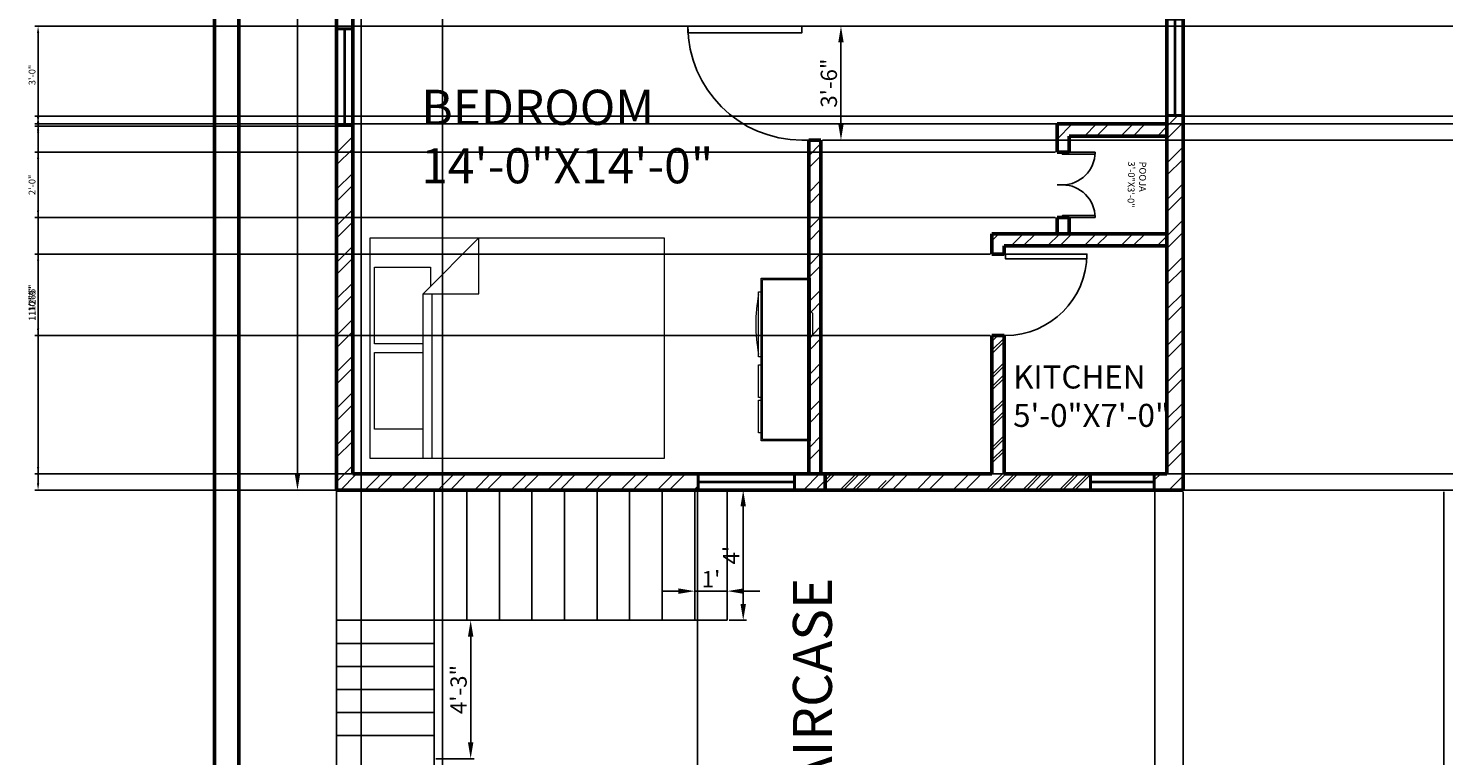
# Model space of a CAD drawing. Units: inches. Extents: x -12550 to 6516, y 1273 to 18700.
# Tile 4 of 19: x 1904 to 2426, y 1958 to 2226. Entities that reach past the tile are written whole.
import ezdxf

# ---------------------------------------------------------------- set-up
doc = ezdxf.new("R2010")
doc.units = ezdxf.units.IN
for name, color, linetype, lineweight in [('A-ANNO-DIMS', 2, 'Continuous', 18), ('A-AREA-IDEN', 1, 'Continuous', 18), ('A-DOOR', 5, 'Continuous', 25), ('A-FLOR-STRS', 6, 'Continuous', 25), ('A-FURN', 8, 'Continuous', 18), ('A-GLAZ', 3, 'Continuous', 25), ('A-WALL', 7, 'Continuous', 50), ('A-WALL-PATT', 8, 'Continuous', 13)]:
    doc.layers.add(name, color=color, linetype=linetype, lineweight=lineweight)
doc.styles.get("Standard").update_dxf_attribs({"font": 'arial.ttf'})
doc.dimstyles.new('ISO-25', dxfattribs={"dimtxt": 2.5, "dimasz": 2.5, "dimexe": 1.25, "dimexo": 0.625, "dimtad": 1, "dimlunit": 4, "dimtxsty": 'Standard', "dimcen": 2.5, "dimadec": 0, "dimazin": 0, "dimtfac": 1, "dimtmove": 0, "dimatfit": 3, "dimfxl": 1, "dimarcsym": 0})
pattern_1 = [(45, (-2e-13, 567), (-6.735192, 6.735192), []), (45, (4.49, 567), (-6.735192, 6.735192), [])]

# ---------------------------------------------------------------- blocks, each defined once
blk = doc.blocks.new('*U2')
for p, q in [((0, 0), (0, -5)), ((30, 0), (30, -5))]:
    blk.add_line(p, q)
blk.add_lwpolyline([(0, 0), (0, 30), (1.75, 30), (1.75, 0)], close=True)
blk.add_arc((0, 0), 30, 0, 90)
blk = doc.blocks.new('Bed - Queen')
for p, q in [((0, -80.00003), (0, 0)), ((0, 0), (59.99999, 0)), ((59.99999, 0), (59.99999, -80.00003)), ((7.99999, -1.2), (28.79998, -1.2)), ((7.99999, -14.4), (7.99999, -1.2)), ((28.79998, -1.2), (28.79998, -14.4)), ((31.19999, -1.2), (51.99999, -1.2)), ((31.19999, -14.4), (31.19999, -1.2)), ((51.99999, -1.2), (51.99999, -16.4)), ((0, -14.4), (44.8, -14.4)), ((59.99999, -29.6), (44.8, -14.4)), ((44.8, -14.4), (44.8, -29.6)), ((44.8, -16.8), (0, -16.8)), ((51.99999, -16.4), (46.79936, -16.4)), ((44.8, -29.6), (59.99999, -29.6)), ((59.99999, -80.00003), (0, -80.00003))]:
    blk.add_line(p, q)
blk = doc.blocks.new('Entertainment Center')
for p, q in [((-4, 0), (-5, -1)), ((4, 0), (-4, 0)), ((5, -1), (4, 0)), ((-17, -19), (-17, -1)), ((-17, -1), (43, -1)), ((-16.5, -18.5), (-16.5, -1.5)), ((-16.5, -1.5), (42.5, -1.5)), ((42.5, -1.5), (42.5, -18.5)), ((43, -1), (43, -19)), ((43, -19), (-17, -19)), ((42.5, -18.5), (-16.5, -18.5)), ((-12, -20), (-12, -19)), ((12, -20), (-12, -20)), ((12, -19), (12, -20)), ((15, -20), (15, -19)), ((27, -20), (15, -20)), ((27, -19), (27, -20)), ((28, -20), (28, -19)), ((40, -20), (28, -20)), ((40, -19), (40, -20))]:
    blk.add_line(p, q)
blk.add_arc((0, 40), 61, 259.6111, 280.3889)
blk = doc.blocks.new('*D10')
at = {"layer": 'A-ANNO-DIMS', "color": 0, "lineweight": -2, "transparency": 16777216}
for p, q in [((2196.81, 2227.25), (2204.82, 2227.25)), ((2203.57, 2221.25), (2203.57, 2191.25)), ((2196.81, 2185.25), (2204.82, 2185.25))]:
    blk.add_line(p, q, dxfattribs=at)
at = {"layer": 'A-ANNO-DIMS', "color": 0, "transparency": 16777216}
for points in [[(2202.57, 2221.25), (2204.57, 2221.25), (2203.57, 2227.25)], [(2202.57, 2191.25), (2204.57, 2191.25), (2203.57, 2185.25)]]:
    blk.add_solid(points, dxfattribs=at)
at = {"layer": 'Defpoints', "color": 0, "transparency": 16777216}
for p in [(2196.19, 2227.25), (2196.19, 2185.25), (2203.57, 2185.25)]:
    blk.add_point(p, dxfattribs=at)
at = {"layer": 'A-ANNO-DIMS', "color": 0, "transparency": 16777216, "insert": (2199.88, 2206.25), "char_height": 6, "attachment_point": 5, "rotation": 90}
blk.add_mtext('3\'-6"', dxfattribs=at)
blk = doc.blocks.new('*D11')
at = {"layer": 'A-ANNO-DIMS', "color": 0, "lineweight": -2, "transparency": 16777216}
for p, q in [((2162.31, 2056.25), (2168.79, 2056.25)), ((2167.54, 2014.25), (2167.54, 2050.25)), ((2162.31, 2008.25), (2168.79, 2008.25))]:
    blk.add_line(p, q, dxfattribs=at)
at = {"layer": 'A-ANNO-DIMS', "color": 0, "transparency": 16777216}
for points in [[(2166.54, 2050.25), (2168.54, 2050.25), (2167.54, 2056.25)], [(2166.54, 2014.25), (2168.54, 2014.25), (2167.54, 2008.25)]]:
    blk.add_solid(points, dxfattribs=at)
at = {"layer": 'Defpoints', "color": 0, "transparency": 16777216}
for p in [(2161.69, 2056.25), (2167.54, 2056.25), (2161.69, 2008.25)]:
    blk.add_point(p, dxfattribs=at)
at = {"layer": 'A-ANNO-DIMS', "color": 0, "transparency": 16777216, "insert": (2163.92, 2032.25), "char_height": 6, "attachment_point": 5, "rotation": 90}
blk.add_mtext("4'", dxfattribs=at)
blk = doc.blocks.new('*D12')
at = {"layer": 'A-ANNO-DIMS', "color": 0, "lineweight": -2, "transparency": 16777216}
for p, q in [((2143.69, 2019.01), (2137.69, 2019.01)), ((2149.69, 2008.87), (2149.69, 2020.26)), ((2161.69, 2019.01), (2149.69, 2019.01)), ((2161.69, 2008.87), (2161.69, 2020.26)), ((2167.69, 2019.01), (2173.69, 2019.01))]:
    blk.add_line(p, q, dxfattribs=at)
at = {"layer": 'A-ANNO-DIMS', "color": 0, "transparency": 16777216}
for points in [[(2143.69, 2020.01), (2143.69, 2018.01), (2149.69, 2019.01)], [(2167.69, 2020.01), (2167.69, 2018.01), (2161.69, 2019.01)]]:
    blk.add_solid(points, dxfattribs=at)
at = {"layer": 'Defpoints', "color": 0, "transparency": 16777216}
for p in [(2149.69, 2019.01), (2149.69, 2008.25), (2161.69, 2008.25)]:
    blk.add_point(p, dxfattribs=at)
at = {"layer": 'A-ANNO-DIMS', "color": 0, "transparency": 16777216, "insert": (2155.69, 2022.65), "char_height": 6, "attachment_point": 5}
blk.add_mtext("1'", dxfattribs=at)
blk = doc.blocks.new('*D13')
at = {"layer": 'A-ANNO-DIMS', "color": 0, "lineweight": -2, "transparency": 16777216}
for p, q in [((2054.31, 2008.25), (2068.36, 2008.25)), ((2067.11, 2002.25), (2067.11, 1963.25)), ((2054.31, 1957.25), (2068.36, 1957.25))]:
    blk.add_line(p, q, dxfattribs=at)
at = {"layer": 'A-ANNO-DIMS', "color": 0, "transparency": 16777216}
for points in [[(2066.11, 2002.25), (2068.11, 2002.25), (2067.11, 2008.25)], [(2066.11, 1963.25), (2068.11, 1963.25), (2067.11, 1957.25)]]:
    blk.add_solid(points, dxfattribs=at)
at = {"layer": 'Defpoints', "color": 0, "transparency": 16777216}
for p in [(2053.69, 2008.25), (2053.69, 1957.25), (2067.11, 1957.25)]:
    blk.add_point(p, dxfattribs=at)
at = {"layer": 'A-ANNO-DIMS', "color": 0, "transparency": 16777216, "insert": (2063.42, 1982.75), "char_height": 6, "attachment_point": 5, "rotation": 90}
blk.add_mtext('4\'-3"', dxfattribs=at)
blk = doc.blocks.new('*D15')
at = {"layer": 'A-ANNO-DIMS', "color": 0, "lineweight": -2, "transparency": 16777216}
for p, q in [((2017.06, 2473.25), (2002.03, 2473.25)), ((2003.28, 2467.25), (2003.28, 2062.25)), ((2017.06, 2056.25), (2002.03, 2056.25))]:
    blk.add_line(p, q, dxfattribs=at)
at = {"layer": 'A-ANNO-DIMS', "color": 0, "transparency": 16777216}
for points in [[(2002.28, 2467.25), (2004.28, 2467.25), (2003.28, 2473.25)], [(2002.28, 2062.25), (2004.28, 2062.25), (2003.28, 2056.25)]]:
    blk.add_solid(points, dxfattribs=at)
at = {"layer": 'Defpoints', "color": 0, "transparency": 16777216}
for p in [(2017.69, 2473.25), (2003.28, 2056.25), (2017.69, 2056.25)]:
    blk.add_point(p, dxfattribs=at)
at = {"layer": 'A-ANNO-DIMS', "color": 0, "transparency": 16777216, "insert": (1999.59, 2264.75), "char_height": 6, "attachment_point": 5, "rotation": 90}
blk.add_mtext('34\'-9"', dxfattribs=at)
blk = doc.blocks.new('WIN-3FT')
for p, q in [((0, 0), (0, 6)), ((0, 6), (36.02, 6)), ((0.5, 0), (0.5, 6)), ((35.52, 6), (35.52, 0)), ((36.02, 6), (36.02, 0)), ((36.02, 0), (0, 0)), ((35.52, 3.2), (0.5, 3.2)), ((35.52, 2.8), (0.5, 2.8))]:
    blk.add_line(p, q)
blk = doc.blocks.new('WIN-2FT')
for p, q in [((0, 0), (0, 24.02)), ((0, 24.02), (6, 24.02)), ((0, 23.52), (6, 23.52)), ((2.8, 0.5), (2.8, 23.52)), ((3.2, 0.5), (3.2, 23.52)), ((6, 24.02), (6, 0)), ((6, 0.5), (0, 0.5)), ((6, 0), (0, 0))]:
    blk.add_line(p, q)
blk = doc.blocks.new('*D133')
at = {"layer": 'A-ANNO-DIMS', "color": 0, "lineweight": -2, "transparency": 16777216}
for p, q in [((2017.06, 2190.44), (1906.44, 2190.44)), ((1907.69, 2058.75), (1907.69, 2187.94)), ((2017.06, 2056.25), (1906.44, 2056.25))]:
    blk.add_line(p, q, dxfattribs=at)
at = {"layer": 'A-ANNO-DIMS', "color": 0, "transparency": 16777216}
for points in [[(1907.27, 2187.94), (1908.11, 2187.94), (1907.69, 2190.44)], [(1907.27, 2058.75), (1908.11, 2058.75), (1907.69, 2056.25)]]:
    blk.add_solid(points, dxfattribs=at)
at = {"layer": 'Defpoints', "color": 0, "transparency": 16777216}
for p in [(1907.69, 2190.44), (2017.69, 2190.44), (2017.69, 2056.25)]:
    blk.add_point(p, dxfattribs=at)
at = {"layer": 'A-ANNO-DIMS', "color": 0, "transparency": 16777216, "insert": (1905.81, 2123.34), "char_height": 2.5, "attachment_point": 5, "rotation": 90}
blk.add_mtext('11\'-2"', dxfattribs=at)
blk = doc.blocks.new('*D136')
at = {"layer": 'A-ANNO-DIMS', "color": 0, "lineweight": -2, "transparency": 16777216}
for p, q in [((2017.69, 2055.62), (2017.69, 1378)), ((2150.64, 2055.62), (2150.64, 1378)), ((2020.19, 1379.25), (2148.14, 1379.25))]:
    blk.add_line(p, q, dxfattribs=at)
at = {"layer": 'A-ANNO-DIMS', "color": 0, "transparency": 16777216}
for points in [[(2020.19, 1379.66), (2020.19, 1378.83), (2017.69, 1379.25)], [(2148.14, 1379.66), (2148.14, 1378.83), (2150.64, 1379.25)]]:
    blk.add_solid(points, dxfattribs=at)
at = {"layer": 'Defpoints', "color": 0, "transparency": 16777216}
for p in [(2017.69, 2056.25), (2150.64, 2056.25), (2150.64, 1379.25)]:
    blk.add_point(p, dxfattribs=at)
at = {"layer": 'A-ANNO-DIMS', "color": 0, "transparency": 16777216, "insert": (2084.16, 1381.13), "char_height": 2.5, "attachment_point": 5}
blk.add_mtext('11\'-1"', dxfattribs=at)
blk = doc.blocks.new('*D137')
at = {"layer": 'A-ANNO-DIMS', "color": 0, "lineweight": -2, "transparency": 16777216}
for p, q in [((2319.29, 2055.62), (2319.29, 1378)), ((2329.69, 2055.62), (2329.69, 1378)), ((2321.79, 1379.25), (2327.19, 1379.25)), ((2329.69, 1379.25), (2347.85, 1379.25))]:
    blk.add_line(p, q, dxfattribs=at)
at = {"layer": 'A-ANNO-DIMS', "color": 0, "transparency": 16777216}
for points in [[(2321.79, 1379.66), (2321.79, 1378.83), (2319.29, 1379.25)], [(2327.19, 1379.66), (2327.19, 1378.83), (2329.69, 1379.25)]]:
    blk.add_solid(points, dxfattribs=at)
at = {"layer": 'Defpoints', "color": 0, "transparency": 16777216}
for p in [(2319.29, 2056.25), (2329.69, 2056.25), (2329.69, 1379.25)]:
    blk.add_point(p, dxfattribs=at)
at = {"layer": 'A-ANNO-DIMS', "color": 0, "transparency": 16777216, "insert": (2340.02, 1381.16), "char_height": 2.5, "attachment_point": 5}
blk.add_mtext('0\'-10 1/2"', dxfattribs=at)
blk = doc.blocks.new('*D138')
at = {"layer": 'A-ANNO-DIMS', "color": 0, "lineweight": -2, "transparency": 16777216}
for p, q in [((2196.81, 2185.25), (2848.94, 2185.25)), ((2847.69, 2064.75), (2847.69, 2182.75)), ((2196.81, 2062.25), (2848.94, 2062.25))]:
    blk.add_line(p, q, dxfattribs=at)
at = {"layer": 'A-ANNO-DIMS', "color": 0, "transparency": 16777216}
for points in [[(2847.27, 2182.75), (2848.11, 2182.75), (2847.69, 2185.25)], [(2847.27, 2064.75), (2848.11, 2064.75), (2847.69, 2062.25)]]:
    blk.add_solid(points, dxfattribs=at)
at = {"layer": 'Defpoints', "color": 0, "transparency": 16777216}
for p in [(2196.19, 2185.25), (2847.69, 2185.25), (2196.19, 2062.25)]:
    blk.add_point(p, dxfattribs=at)
at = {"layer": 'A-ANNO-DIMS', "color": 0, "transparency": 16777216, "insert": (2845.79, 2123.75), "char_height": 2.5, "attachment_point": 5, "rotation": 90}
blk.add_mtext('10\'-3"', dxfattribs=at)
blk = doc.blocks.new('*D142')
at = {"layer": 'A-ANNO-DIMS', "color": 0, "lineweight": -2, "transparency": 16777216}
for p, q in [((2026.69, 2234.12), (2026.69, 1378)), ((2056.69, 2234.12), (2056.69, 1378)), ((2029.19, 1379.25), (2054.19, 1379.25))]:
    blk.add_line(p, q, dxfattribs=at)
at = {"layer": 'A-ANNO-DIMS', "color": 0, "transparency": 16777216}
for points in [[(2029.19, 1379.66), (2029.19, 1378.83), (2026.69, 1379.25)], [(2054.19, 1379.66), (2054.19, 1378.83), (2056.69, 1379.25)]]:
    blk.add_solid(points, dxfattribs=at)
at = {"layer": 'Defpoints', "color": 0, "transparency": 16777216}
for p in [(2026.69, 2234.75), (2056.69, 2234.75), (2056.69, 1379.25)]:
    blk.add_point(p, dxfattribs=at)
at = {"layer": 'A-ANNO-DIMS', "color": 0, "transparency": 16777216, "insert": (2041.69, 1381.15), "char_height": 2.5, "attachment_point": 5}
blk.add_mtext('2\'-6"', dxfattribs=at)
blk = doc.blocks.new('*D145')
at = {"layer": 'A-ANNO-DIMS', "color": 0, "lineweight": -2, "transparency": 16777216}
for p, q in [((2330.31, 2194.03), (2848.94, 2194.03)), ((2847.69, 2058.75), (2847.69, 2191.53)), ((2330.31, 2056.25), (2848.94, 2056.25))]:
    blk.add_line(p, q, dxfattribs=at)
at = {"layer": 'A-ANNO-DIMS', "color": 0, "transparency": 16777216}
for points in [[(2847.27, 2191.53), (2848.11, 2191.53), (2847.69, 2194.03)], [(2847.27, 2058.75), (2848.11, 2058.75), (2847.69, 2056.25)]]:
    blk.add_solid(points, dxfattribs=at)
at = {"layer": 'Defpoints', "color": 0, "transparency": 16777216}
for p in [(2329.69, 2194.03), (2847.69, 2194.03), (2329.69, 2056.25)]:
    blk.add_point(p, dxfattribs=at)
at = {"layer": 'A-ANNO-DIMS', "color": 0, "transparency": 16777216, "insert": (2845.79, 2125.14), "char_height": 2.5, "attachment_point": 5, "rotation": 90}
blk.add_mtext('11\'-6"', dxfattribs=at)
blk = doc.blocks.new('*D147')
at = {"layer": 'A-ANNO-DIMS', "color": 0, "lineweight": -2, "transparency": 16777216}
for p, q in [((2258.56, 2143.25), (1906.44, 2143.25)), ((1907.69, 2115.75), (1907.69, 2140.75)), ((2258.56, 2113.25), (1906.44, 2113.25))]:
    blk.add_line(p, q, dxfattribs=at)
at = {"layer": 'A-ANNO-DIMS', "color": 0, "transparency": 16777216}
for points in [[(1907.27, 2140.75), (1908.11, 2140.75), (1907.69, 2143.25)], [(1907.27, 2115.75), (1908.11, 2115.75), (1907.69, 2113.25)]]:
    blk.add_solid(points, dxfattribs=at)
at = {"layer": 'Defpoints', "color": 0, "transparency": 16777216}
for p in [(1907.69, 2143.25), (2259.19, 2143.25), (2259.19, 2113.25)]:
    blk.add_point(p, dxfattribs=at)
at = {"layer": 'A-ANNO-DIMS', "color": 0, "transparency": 16777216, "insert": (1905.79, 2128.25), "char_height": 2.5, "attachment_point": 5, "rotation": 90}
blk.add_mtext('2\'-6"', dxfattribs=at)
blk = doc.blocks.new('*D148')
at = {"layer": 'A-ANNO-DIMS', "color": 0, "lineweight": -2, "transparency": 16777216}
for p, q in [((2282.56, 2180.75), (1906.44, 2180.75)), ((1907.69, 2159.25), (1907.69, 2178.25)), ((2282.56, 2156.75), (1906.44, 2156.75))]:
    blk.add_line(p, q, dxfattribs=at)
at = {"layer": 'A-ANNO-DIMS', "color": 0, "transparency": 16777216}
for points in [[(1907.27, 2178.25), (1908.11, 2178.25), (1907.69, 2180.75)], [(1907.27, 2159.25), (1908.11, 2159.25), (1907.69, 2156.75)]]:
    blk.add_solid(points, dxfattribs=at)
at = {"layer": 'Defpoints', "color": 0, "transparency": 16777216}
for p in [(1907.69, 2180.75), (2283.19, 2180.75), (2283.19, 2156.75)]:
    blk.add_point(p, dxfattribs=at)
at = {"layer": 'A-ANNO-DIMS', "color": 0, "transparency": 16777216, "insert": (1905.79, 2168.75), "char_height": 2.5, "attachment_point": 5, "rotation": 90}
blk.add_mtext('2\'-0"', dxfattribs=at)
blk = doc.blocks.new('*D152')
at = {"layer": 'A-ANNO-DIMS', "color": 0, "lineweight": -2, "transparency": 16777216}
for p, q in [((2425.69, 2055.62), (2425.69, 1378)), ((2500.53, 2055.62), (2500.53, 1378)), ((2428.19, 1379.25), (2498.03, 1379.25))]:
    blk.add_line(p, q, dxfattribs=at)
at = {"layer": 'A-ANNO-DIMS', "color": 0, "transparency": 16777216}
for points in [[(2428.19, 1379.66), (2428.19, 1378.83), (2425.69, 1379.25)], [(2498.03, 1379.66), (2498.03, 1378.83), (2500.53, 1379.25)]]:
    blk.add_solid(points, dxfattribs=at)
at = {"layer": 'Defpoints', "color": 0, "transparency": 16777216}
for p in [(2425.69, 2056.25), (2500.53, 2056.25), (2500.53, 1379.25)]:
    blk.add_point(p, dxfattribs=at)
at = {"layer": 'A-ANNO-DIMS', "color": 0, "transparency": 16777216, "insert": (2463.11, 1381.15), "char_height": 2.5, "attachment_point": 5}
blk.add_mtext('6\'-3"', dxfattribs=at)
blk = doc.blocks.new('*D157')
at = {"layer": 'A-ANNO-DIMS', "color": 0, "lineweight": -2, "transparency": 16777216}
for p, q in [((2558.56, 2191.25), (1906.44, 2191.25)), ((1907.69, 2064.75), (1907.69, 2188.75)), ((2558.56, 2062.25), (1906.44, 2062.25))]:
    blk.add_line(p, q, dxfattribs=at)
at = {"layer": 'A-ANNO-DIMS', "color": 0, "transparency": 16777216}
for points in [[(1907.27, 2188.75), (1908.11, 2188.75), (1907.69, 2191.25)], [(1907.27, 2064.75), (1908.11, 2064.75), (1907.69, 2062.25)]]:
    blk.add_solid(points, dxfattribs=at)
at = {"layer": 'Defpoints', "color": 0, "transparency": 16777216}
for p in [(1907.69, 2191.25), (2559.19, 2191.25), (2559.19, 2062.25)]:
    blk.add_point(p, dxfattribs=at)
at = {"layer": 'A-ANNO-DIMS', "color": 0, "transparency": 16777216, "insert": (1905.79, 2126.75), "char_height": 2.5, "attachment_point": 5, "rotation": 90}
blk.add_mtext('10\'-9"', dxfattribs=at)
blk = doc.blocks.new('*D158')
at = {"layer": 'A-ANNO-DIMS', "color": 0, "lineweight": -2, "transparency": 16777216}
for p, q in [((2558.56, 2227.25), (1906.44, 2227.25)), ((1907.69, 2193.75), (1907.69, 2224.75)), ((2558.56, 2191.25), (1906.44, 2191.25))]:
    blk.add_line(p, q, dxfattribs=at)
at = {"layer": 'A-ANNO-DIMS', "color": 0, "transparency": 16777216}
for points in [[(1907.27, 2224.75), (1908.11, 2224.75), (1907.69, 2227.25)], [(1907.27, 2193.75), (1908.11, 2193.75), (1907.69, 2191.25)]]:
    blk.add_solid(points, dxfattribs=at)
at = {"layer": 'Defpoints', "color": 0, "transparency": 16777216}
for p in [(1907.69, 2227.25), (2559.19, 2227.25), (2559.19, 2191.25)]:
    blk.add_point(p, dxfattribs=at)
at = {"layer": 'A-ANNO-DIMS', "color": 0, "transparency": 16777216, "insert": (1905.79, 2209.25), "char_height": 2.5, "attachment_point": 5, "rotation": 90}
blk.add_mtext('3\'-0"', dxfattribs=at)
blk = doc.blocks.new('*D165')
at = {"layer": 'A-ANNO-DIMS', "color": 0, "lineweight": -2, "transparency": 16777216}
for p, q in [((2425.06, 2194.03), (1906.44, 2194.03)), ((1907.69, 2058.75), (1907.69, 2191.53)), ((2425.06, 2056.25), (1906.44, 2056.25))]:
    blk.add_line(p, q, dxfattribs=at)
at = {"layer": 'A-ANNO-DIMS', "color": 0, "transparency": 16777216}
for points in [[(1907.27, 2191.53), (1908.11, 2191.53), (1907.69, 2194.03)], [(1907.27, 2058.75), (1908.11, 2058.75), (1907.69, 2056.25)]]:
    blk.add_solid(points, dxfattribs=at)
at = {"layer": 'Defpoints', "color": 0, "transparency": 16777216}
for p in [(1907.69, 2194.03), (2425.69, 2194.03), (2425.69, 2056.25)]:
    blk.add_point(p, dxfattribs=at)
at = {"layer": 'A-ANNO-DIMS', "color": 0, "transparency": 16777216, "insert": (1905.79, 2125.14), "char_height": 2.5, "attachment_point": 5, "rotation": 90}
blk.add_mtext('11\'-6"', dxfattribs=at)

msp = doc.modelspace()

# ---------------------------------------------------------------- hatches: boundary and pattern name
at = {"layer": 'A-WALL-PATT'}
h = msp.add_hatch(dxfattribs=at)
h.set_pattern_fill('ANSI32', color=256)
h.set_pattern_definition(pattern_1)
h.paths.add_polyline_path([(2023.689, 2255.449), (2017.689, 2255.449), (2017.689, 2226.453), (2023.689, 2226.453), (2023.689, 2230.247), (2026.689, 2230.247), (2026.689, 2234.747), (2023.689, 2234.747)])
h = msp.add_hatch(dxfattribs=at)
h.set_pattern_fill('ANSI32', color=256)
h.set_pattern_definition(pattern_1)
h.paths.add_polyline_path([(2323.689, 2191.247), (2283.189, 2191.247), (2283.189, 2180.747), (2285.189, 2180.747), (2287.689, 2180.747), (2287.689, 2186.747), (2323.689, 2186.747)])
h = msp.add_hatch(dxfattribs=at)
h.set_pattern_fill('ANSI32', color=256)
h.set_pattern_definition(pattern_1)
h.paths.add_polyline_path([(2329.689, 2194.032), (2323.689, 2194.032), (2323.689, 2062.247), (2319.294, 2062.247), (2319.294, 2056.247), (2329.689, 2056.247)])
h = msp.add_hatch(dxfattribs=at)
h.set_pattern_fill('ANSI32', color=256)
h.set_pattern_definition(pattern_1)
h.paths.add_polyline_path([(2023.689, 2190.435), (2017.689, 2190.435), (2017.689, 2056.247), (2150.64, 2056.247), (2150.64, 2062.247), (2023.689, 2062.247)])
h = msp.add_hatch(dxfattribs=at)
h.set_pattern_fill('ANSI32', color=256)
h.set_pattern_definition(pattern_1)
h.paths.add_polyline_path([(2196.189, 2185.247), (2191.689, 2185.247), (2191.689, 2134.365), (2192.189, 2134.365), (2192.189, 2122.365), (2193.189, 2121.365), (2193.189, 2113.365), (2192.189, 2112.365), (2192.189, 2074.365), (2191.689, 2062.247), (2196.189, 2062.247)])
h = msp.add_hatch(dxfattribs=at)
h.set_pattern_fill('ANSI32', color=256)
h.set_pattern_definition(pattern_1)
h.paths.add_polyline_path([(2323.689, 2150.747), (2259.189, 2150.747), (2259.189, 2143.247), (2263.689, 2143.247), (2263.689, 2146.247), (2323.689, 2146.247)])
h = msp.add_hatch(dxfattribs=at)
h.set_pattern_fill('ANSI32', color=256)
h.paths.add_polyline_path([(2295.277, 2062.247), (2263.689, 2062.247), (2263.689, 2113.247), (2259.189, 2113.247), (2259.189, 2062.247), (2256.189, 2062.247), (2197.689, 2062.247), (2197.689, 2056.247), (2256.189, 2056.247), (2295.277, 2056.247)])
h = msp.add_hatch(dxfattribs=at)
h.set_pattern_fill('ANSI32', color=256)
h.set_pattern_definition(pattern_1)
h.paths.add_polyline_path([(2263.689, 2062.247), (2263.689, 2113.247), (2259.189, 2113.247), (2259.189, 2062.247), (2256.189, 2062.247), (2256.189, 2056.247), (2295.277, 2056.247), (2295.277, 2062.247)])
h = msp.add_hatch(dxfattribs=at)
h.set_pattern_fill('ANSI32', color=256)
h.set_pattern_definition(pattern_1)
h.paths.add_polyline_path([(2186.657, 2062.247), (2186.657, 2056.247), (2220.189, 2056.247), (2220.189, 2062.247)])

# ---------------------------------------------------------------- linework, layer by layer
at = {"layer": 'A-FLOR-STRS'}
for p, q in [((2197.689, 2056.247), (2017.689, 2056.247)), ((2017.689, 2056.247), (2017.689, 1906.247)), ((2053.689, 2056.247), (2053.689, 1906.247)), ((2065.689, 2056.247), (2065.689, 2008.247)), ((2077.689, 2056.247), (2077.689, 2008.247)), ((2089.689, 2056.247), (2089.689, 2008.247)), ((2101.689, 2056.247), (2101.689, 2008.247)), ((2113.689, 2056.247), (2113.689, 2008.247)), ((2125.689, 2056.247), (2125.689, 2008.247)), ((2137.689, 2056.247), (2137.689, 2008.247)), ((2149.689, 2056.247), (2149.689, 2008.247)), ((2161.689, 2056.247), (2161.689, 2008.247)), ((2017.689, 2008.247), (2161.689, 2008.247)), ((2017.689, 2008.247), (2161.689, 2008.247)), ((2017.689, 1999.747), (2053.689, 1999.747)), ((2017.689, 1991.247), (2053.689, 1991.247)), ((2017.689, 1982.747), (2053.689, 1982.747)), ((2017.689, 1974.247), (2053.689, 1974.247)), ((2017.689, 1965.747), (2053.689, 1965.747))]:
    msp.add_line(p, q, dxfattribs=at)
at = {"layer": 'A-WALL'}
for p, q in [((1972.689, 1444.247), (1972.689, 2518.247)), ((1981.689, 1453.247), (1981.689, 2509.247)), ((2017.689, 2068.324), (2017.689, 2473.247)), ((2323.689, 2062.247), (2323.689, 2234.747)), ((2329.689, 2056.247), (2329.689, 2234.747)), ((2023.689, 2062.247), (2023.689, 2230.247)), ((2323.689, 2191.247), (2283.189, 2191.247)), ((2283.189, 2180.747), (2283.189, 2191.247)), ((2323.689, 2186.747), (2287.689, 2186.747)), ((2287.689, 2180.747), (2287.689, 2186.747)), ((2191.689, 2062.247), (2191.689, 2185.247)), ((2191.689, 2185.247), (2196.189, 2185.247)), ((2196.189, 2062.247), (2196.189, 2185.247)), ((2283.189, 2180.747), (2287.689, 2180.747)), ((2283.189, 2150.747), (2283.189, 2156.747)), ((2287.689, 2156.747), (2283.189, 2156.747)), ((2283.189, 2150.747), (2283.189, 2155.747)), ((2287.689, 2150.747), (2287.689, 2156.747)), ((2287.689, 2150.747), (2287.689, 2156.747)), ((2323.689, 2150.747), (2259.189, 2150.747)), ((2259.189, 2143.247), (2259.189, 2150.747)), ((2323.689, 2146.247), (2263.689, 2146.247)), ((2263.689, 2143.247), (2263.689, 2146.247)), ((2263.689, 2146.247), (2263.689, 2143.247)), ((2263.689, 2143.247), (2259.189, 2143.247)), ((2259.189, 2062.247), (2259.189, 2113.247)), ((2259.189, 2113.247), (2263.689, 2113.247)), ((2263.689, 2062.247), (2263.689, 2113.247)), ((2017.689, 2056.247), (2017.689, 2068.324)), ((2256.189, 2062.247), (2023.689, 2062.247)), ((2220.189, 2062.247), (2196.189, 2062.247)), ((2197.689, 2056.247), (2197.689, 2062.247)), ((2259.189, 2062.247), (2256.189, 2062.247)), ((2259.189, 2062.247), (2256.189, 2062.247)), ((2323.689, 2062.247), (2263.689, 2062.247)), ((2256.189, 2056.247), (2017.689, 2056.247)), ((2329.689, 2056.247), (2256.189, 2056.247))]:
    msp.add_line(p, q, dxfattribs=at)

# ---------------------------------------------------------------- block references
at = {"layer": 'A-DOOR'}
for p, xscale, yscale, zscale, rotation in [((2189.189, 2227.247), -1.4, 1.4, 1.4, 90), ((2285.189, 2180.747), 0.399999999999997, 0.399999999999997, 0.399999999999997, 270), ((2285.189, 2156.747), -0.399999999999997, 0.399999999999997, 0.399999999999997, 270)]:
    msp.add_blockref('*U2', p, dxfattribs=dict(at, xscale=xscale, yscale=yscale, zscale=zscale, rotation=rotation))
at = {"layer": 'A-DOOR', "rotation": 270}
msp.add_blockref('*U2', (2264.189, 2143.247), dxfattribs=at)
at = {"layer": 'A-FURN', "xscale": 1.354827908062564, "yscale": 1.354827908062564, "zscale": 1.354827908062564, "rotation": 90}
msp.add_blockref('Bed - Queen', (2030.038, 2067.915), dxfattribs=at)
at = {"layer": 'A-FURN', "rotation": 270}
msp.add_blockref('Entertainment Center', (2193.189, 2117.365), dxfattribs=at)
at = {"layer": 'A-GLAZ'}
for name, p, rotation in [('WIN-3FT', (2329.689, 2194.032), 90.00000000000188), ('WIN-3FT', (2023.689, 2190.436), 89.9999999999993), ('WIN-3FT', (2186.657, 2062.247), 180), ('WIN-2FT', (2295.276, 2062.247), 269.9999999999985)]:
    msp.add_blockref(name, p, dxfattribs=dict(at, rotation=rotation))

# ---------------------------------------------------------------- texts
at = {"layer": 'A-AREA-IDEN', "insert": (2048.907, 2203.812), "char_height": 12.93169, "attachment_point": 1}
msp.add_mtext('BEDROOM\\P14\'-0"X14\'-0"', dxfattribs=at)
at = {"layer": 'A-AREA-IDEN', "attachment_point": 1}
for s, width, gutter_width, insert, char_height, rotation in [('POOJA\\P3\'-0"X3\'-0"', 0.78585, 12.5, (2316.065, 2177.304), 2.5, 269.18385), ('STAIRCASE', 2.19144, 71.795, (2185.866, 1922.837), 14.3589, 90)]:
    msp.add_mtext_dynamic_manual_height_columns(s, width=width, gutter_width=gutter_width, heights=[0], dxfattribs=dict(at, insert=insert, char_height=char_height, rotation=rotation))
at = {"layer": 'A-AREA-IDEN', "insert": (2267.01, 2102.176), "char_height": 8.48435, "attachment_point": 1}
msp.add_mtext_dynamic_manual_height_columns('KITCHEN\\P5\'-0"X7\'-0"', width=1.29487, gutter_width=42.422, heights=[0], dxfattribs=at)

# ---------------------------------------------------------------- dimensions: what is measured, and where the dimension line sits
at = {"layer": 'A-ANNO-DIMS'}
for base, p1, p2, override, picture, middle in [((2003.28, 2056.247), (2017.689, 2473.247), (2017.689, 2056.247), {"dimtxt": 6, "dimasz": 6, "dimclrd": 0, "dimclre": 0, "dimclrt": 0}, '*D15', (1999.59, 2264.747)), ((1907.689, 2227.247), (2559.189, 2191.247), (2559.189, 2227.247), {"dimdec": 1, "dimlfac": 1, "dimrnd": 0, "dimzin": 1, "dimdsep": 46, "dimlunit": 4, "dimfrac": 2}, '*D158', (1905.787, 2209.247)), ((2203.572, 2185.247), (2196.189, 2227.247), (2196.189, 2185.247), {"dimtxt": 6, "dimasz": 6, "dimclrd": 0, "dimclre": 0, "dimclrt": 0}, '*D10', (2199.882, 2206.247)), ((1907.689, 2194.032), (2425.689, 2056.247), (2425.689, 2194.032), {"dimdec": 1, "dimlfac": 1, "dimrnd": 0, "dimzin": 1, "dimdsep": 46, "dimlunit": 4, "dimfrac": 2}, '*D165', (1905.787, 2125.14)), ((1907.689, 2191.247), (2559.189, 2062.247), (2559.189, 2191.247), {"dimdec": 1, "dimlfac": 1, "dimrnd": 0, "dimzin": 1, "dimdsep": 46, "dimlunit": 4, "dimfrac": 2}, '*D157', (1905.787, 2126.747)), ((2847.689, 2194.032), (2329.689, 2056.247), (2329.689, 2194.032), {"dimdec": 1, "dimlfac": 1, "dimrnd": 0, "dimzin": 1, "dimdsep": 46, "dimlunit": 4, "dimfrac": 2}, '*D145', (2845.787, 2125.14)), ((1907.689, 2190.435), (2017.689, 2056.247), (2017.689, 2190.435), {"dimdec": 1, "dimlfac": 1, "dimrnd": 0, "dimzin": 1, "dimdsep": 46, "dimlunit": 4, "dimfrac": 2}, '*D133', (1905.809, 2123.341)), ((1907.689, 2180.747), (2283.189, 2156.747), (2283.189, 2180.747), {"dimdec": 1, "dimlfac": 1, "dimrnd": 0, "dimzin": 1, "dimdsep": 46, "dimlunit": 4, "dimfrac": 2}, '*D148', (1905.787, 2168.747)), ((2847.689, 2185.247), (2196.189, 2062.247), (2196.189, 2185.247), {"dimdec": 1, "dimlfac": 1, "dimrnd": 0, "dimzin": 1, "dimdsep": 46, "dimlunit": 4, "dimfrac": 2}, '*D138', (2845.787, 2123.747)), ((1907.689, 2143.247), (2259.189, 2113.247), (2259.189, 2143.247), {"dimdec": 1, "dimlfac": 1, "dimrnd": 0, "dimzin": 1, "dimdsep": 46, "dimlunit": 4, "dimfrac": 2}, '*D147', (1905.787, 2128.247)), ((2167.541, 2056.247), (2161.689, 2008.247), (2161.689, 2056.247), {"dimtxt": 6, "dimasz": 6, "dimclrd": 0, "dimclre": 0, "dimclrt": 0}, '*D11', (2163.916, 2032.247)), ((2067.111, 1957.247), (2053.689, 2008.247), (2053.689, 1957.247), {"dimtxt": 6, "dimasz": 6, "dimclrd": 0, "dimclre": 0, "dimclrt": 0}, '*D13', (2063.42, 1982.747))]:
    dim = msp.add_linear_dim(base=base, p1=p1, p2=p2, angle=90, dimstyle='ISO-25', override=override, dxfattribs=at)
    dim.commit()
    dim.dimension.update_dxf_attribs({"geometry": picture, "text_midpoint": middle})
for base, p1, p2, override, picture, middle in [((2056.689, 1379.247), (2026.689, 2234.747), (2056.689, 2234.747), {"dimdec": 1, "dimlfac": 1, "dimrnd": 0, "dimzin": 1, "dimdsep": 46, "dimlunit": 4, "dimfrac": 2}, '*D142', (2041.689, 1381.149)), ((2150.64, 1379.247), (2017.689, 2056.247), (2150.64, 2056.247), {"dimdec": 1, "dimlfac": 1, "dimrnd": 0, "dimzin": 1, "dimdsep": 46, "dimlunit": 4, "dimfrac": 2}, '*D136', (2084.164, 1381.127)), ((2329.689, 1379.247), (2319.294, 2056.247), (2329.689, 2056.247), {"dimdec": 1, "dimlfac": 1, "dimrnd": 0, "dimzin": 1, "dimdsep": 46, "dimlunit": 4, "dimfrac": 2}, '*D137', (2340.02, 1381.165)), ((2500.528, 1379.247), (2425.689, 2056.247), (2500.528, 2056.247), {"dimdec": 1, "dimlfac": 1, "dimrnd": 0, "dimzin": 1, "dimdsep": 46, "dimlunit": 4, "dimfrac": 2}, '*D152', (2463.108, 1381.15)), ((2149.689, 2019.012), (2161.689, 2008.247), (2149.689, 2008.247), {"dimtxt": 6, "dimasz": 6, "dimclrd": 0, "dimclre": 0, "dimclrt": 0}, '*D12', (2155.689, 2022.65))]:
    dim = msp.add_linear_dim(base=base, p1=p1, p2=p2, dimstyle='ISO-25', override=override, dxfattribs=at)
    dim.commit()
    dim.dimension.update_dxf_attribs({"geometry": picture, "text_midpoint": middle})

doc.saveas('drawing.dxf')
